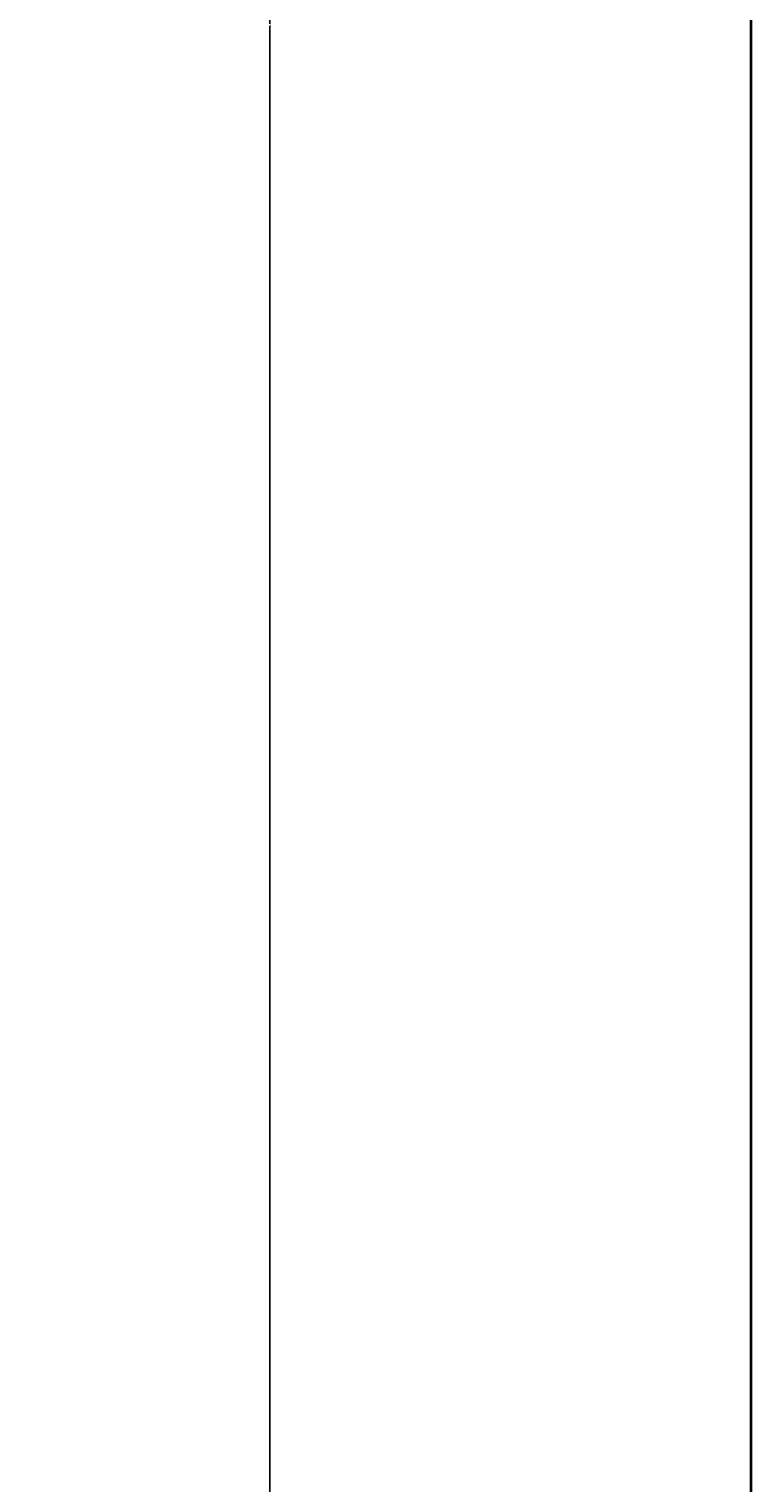
# Model space of a CAD drawing. Units: inches. Extents: x 1513 to 2170, y 1240 to 2288.
# Tile 6 of 10: x 2045 to 2170, y 1549 to 1801. Entities that reach past the tile are written whole.
import ezdxf

# ---------------------------------------------------------------- set-up
doc = ezdxf.new("R2010")
doc.units = ezdxf.units.IN
doc.layers.add('A-ANNO-DIMS', color=2, linetype='Continuous', lineweight=18)
doc.layers.add('A-ANNO-TTLB', color=7, linetype='Continuous', lineweight=35)
doc.styles.get("Standard").update_dxf_attribs({"font": 'arial.ttf'})
doc.dimstyles.get("Standard").update_dxf_attribs({"dimtxt": 0.18, "dimasz": 0.18, "dimexe": 0.18, "dimexo": 0.0625, "dimgap": 0.09, "dimtad": 0, "dimtih": 1, "dimtoh": 1, "dimdec": 4, "dimzin": 0, "dimdsep": 46, "dimtxsty": 'Standard', "dimcen": 0.09, "dimadec": 0, "dimazin": 0, "dimtfac": 1, "dimtdec": 4, "dimtofl": 0, "dimtmove": 0, "dimatfit": 3, "dimfxl": 1, "dimtolj": 1, "dimtzin": 0, "dimarcsym": 0})

# ---------------------------------------------------------------- blocks, each defined once
blk = doc.blocks.new('*D26')
at = {"layer": 'A-ANNO-DIMS', "color": 0, "lineweight": -2, "transparency": 16777216}
for p, q in [((2014.91, 2214.48), (2087.18, 2214.48)), ((2087, 2214.3), (2087, 1802.16)), ((2087, 1389.66), (2087, 1801.8)), ((1937.43, 1389.48), (2087.18, 1389.48))]:
    blk.add_line(p, q, dxfattribs=at)
at = {"layer": 'A-ANNO-DIMS', "color": 0, "transparency": 16777216}
for points in [[(2086.97, 2214.3), (2087.03, 2214.3), (2087, 2214.48)], [(2086.97, 1389.66), (2087.03, 1389.66), (2087, 1389.48)]]:
    blk.add_solid(points, dxfattribs=at)
at = {"layer": 'Defpoints', "color": 0, "transparency": 16777216}
for p in [(2014.85, 2214.48), (2087, 2214.48), (1937.37, 1389.48)]:
    blk.add_point(p, dxfattribs=at)
at = {"layer": 'A-ANNO-DIMS', "color": 0, "transparency": 16777216, "insert": (2087, 1801.98), "char_height": 0.18, "attachment_point": 5}
blk.add_mtext('\\A1;825', dxfattribs=at)

msp = doc.modelspace()

# ---------------------------------------------------------------- linework, layer by layer
at = {"layer": 'A-ANNO-TTLB'}
msp.add_lwpolyline([(1513.071, 2287.731), (2170.435, 2287.731), (2170.435, 1239.669), (1513.071, 1239.669)], close=True, dxfattribs=at)

# ---------------------------------------------------------------- dimensions: what is measured, and where the dimension line sits
at = {"layer": 'A-ANNO-DIMS'}
dim = msp.add_linear_dim(base=(2087.002, 2214.48), p1=(1937.366, 1389.48), p2=(2014.852, 2214.48), angle=90, dimstyle='Standard', override={"dimdec": 0, "dimlfac": 1, "dimrnd": 0, "dimzin": 0, "dimdsep": 46, "dimlunit": 2}, dxfattribs=at)
dim.commit()
dim.dimension.update_dxf_attribs({"geometry": '*D26', "text_midpoint": (2087.002, 1801.98)})

doc.saveas('drawing.dxf')
